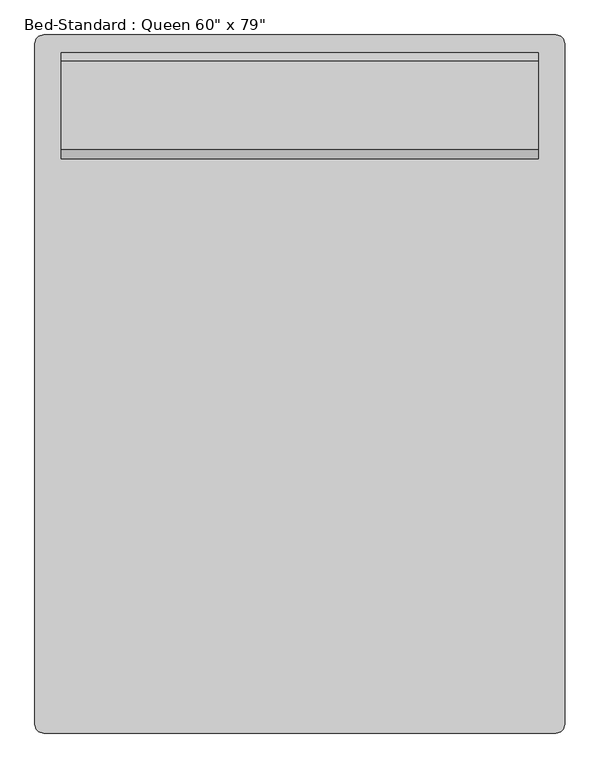
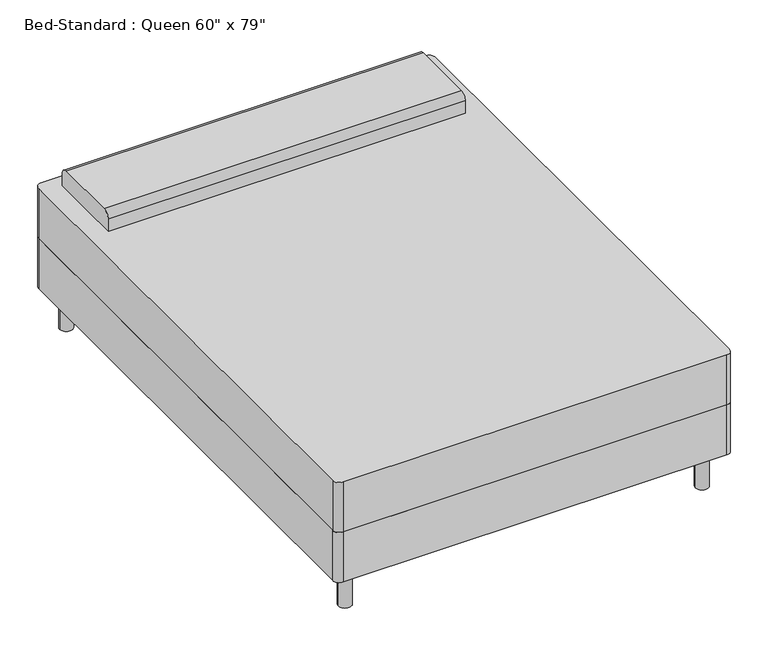
"""IFC4 building model written with IfcOpenShell, lengths in millimetres: furniture geometry."""

from ifc_helpers import new_model, si_unit, point, frame, frame_2d, origin, origin_with_axes, place, context, project, spatial, polyline, circle_curve, trimmed, segment, composite_curve, outline, extrude, source, transform, mapped, element, save


def furniture_e1791683(model_context):
    return source(origin(), model_context, "Body", "SweptSolid", [
        extrude(outline(composite_curve([segment(polyline([(-490.5114754, -1023.495082), (-490.5114754, 932.304918)]), True, "CONTINUOUS"), segment(trimmed(circle_curve(frame_2d((-465.1114754, 932.304918)), 25.4), [point((-490.5114754, 932.304918))], [point((-465.1114754, 957.704918))], False, "CARTESIAN"), True, "CONTINUOUS"), segment(polyline([(-465.1114754, 957.704918), (1008.0885246, 957.704918)]), True, "CONTINUOUS"), segment(trimmed(circle_curve(frame_2d((1008.0885246, 932.304918)), 25.4), [point((1008.0885246, 957.704918))], [point((1033.4885246, 932.304918))], False, "CARTESIAN"), True, "CONTINUOUS"), segment(polyline([(1033.4885246, 932.304918), (1033.4885246, -1023.495082)]), True, "CONTINUOUS"), segment(trimmed(circle_curve(frame_2d((1008.0885246, -1023.495082)), 25.4), [point((1033.4885246, -1023.495082))], [point((1008.0885246, -1048.895082))], False, "CARTESIAN"), True, "CONTINUOUS"), segment(polyline([(1008.0885246, -1048.895082), (-465.1114754, -1048.895082)]), True, "CONTINUOUS"), segment(trimmed(circle_curve(frame_2d((-465.1114754, -1023.495082)), 25.4), [point((-465.1114754, -1048.895082))], [point((-490.5114754, -1023.495082))], False, "CARTESIAN"), True, "CONTINUOUS")], self_intersect=False)), frame((0.0, 0.0, 152.4), z_axis=(0.0, 0.0, 1.0), x_axis=(1.0, 0.0, 0.0)), (0.0, 0.0, 1.0), 203.2),
        extrude(outline(composite_curve([segment(polyline([(602.104918, 558.8), (602.104918, 609.6)]), True, "CONTINUOUS"), segment(trimmed(circle_curve(frame_2d((627.504918, 609.6)), 25.4), [point((602.104918, 609.6))], [point((627.504918, 635.0))], False, "CARTESIAN"), True, "CONTINUOUS"), segment(polyline([(627.504918, 635.0), (881.504918, 635.0)]), True, "CONTINUOUS"), segment(trimmed(circle_curve(frame_2d((881.504918, 609.6)), 25.4), [point((881.504918, 635.0))], [point((906.904918, 609.6))], False, "CARTESIAN"), True, "CONTINUOUS"), segment(polyline([(906.904918, 609.6), (906.904918, 558.8), (602.104918, 558.8)]), True, "CONTINUOUS")], self_intersect=False)), frame((-414.3114754, 0.0, 0.0), z_axis=(1.0, 0.0, 0.0), x_axis=(0.0, 1.0, 0.0)), (0.0, 0.0, 1.0), 1371.6),
        extrude(outline(composite_curve([segment(trimmed(circle_curve(frame_2d((-414.3114754, 881.504918)), 25.4), [point((-439.7114754, 881.504918))], [point((-388.9114754, 881.504918))], False, "CARTESIAN"), True, "CONTINUOUS"), segment(trimmed(circle_curve(frame_2d((-414.3114754, 881.504918)), 25.4), [point((-388.9114754, 881.504918))], [point((-439.7114754, 881.504918))], False, "CARTESIAN"), True, "CONTINUOUS")], self_intersect=False)), origin_with_axes(), (0.0, 0.0, 1.0), 152.4),
        extrude(outline(composite_curve([segment(trimmed(circle_curve(frame_2d((957.2885246, 881.504918)), 25.4), [point((931.8885246, 881.504918))], [point((982.6885246, 881.504918))], False, "CARTESIAN"), True, "CONTINUOUS"), segment(trimmed(circle_curve(frame_2d((957.2885246, 881.504918)), 25.4), [point((982.6885246, 881.504918))], [point((931.8885246, 881.504918))], False, "CARTESIAN"), True, "CONTINUOUS")], self_intersect=False)), origin_with_axes(), (0.0, 0.0, 1.0), 152.4),
        extrude(outline(composite_curve([segment(trimmed(circle_curve(frame_2d((957.2885246, -972.695082)), 25.4), [point((931.8885246, -972.695082))], [point((982.6885246, -972.695082))], False, "CARTESIAN"), True, "CONTINUOUS"), segment(trimmed(circle_curve(frame_2d((957.2885246, -972.695082)), 25.4), [point((982.6885246, -972.695082))], [point((931.8885246, -972.695082))], False, "CARTESIAN"), True, "CONTINUOUS")], self_intersect=False)), origin_with_axes(), (0.0, 0.0, 1.0), 152.4),
        extrude(outline(composite_curve([segment(trimmed(circle_curve(frame_2d((-414.3114754, -972.695082)), 25.4), [point((-439.7114754, -972.695082))], [point((-388.9114754, -972.695082))], False, "CARTESIAN"), True, "CONTINUOUS"), segment(trimmed(circle_curve(frame_2d((-414.3114754, -972.695082)), 25.4), [point((-388.9114754, -972.695082))], [point((-439.7114754, -972.695082))], False, "CARTESIAN"), True, "CONTINUOUS")], self_intersect=False)), origin_with_axes(), (0.0, 0.0, 1.0), 152.4),
        extrude(outline(composite_curve([segment(polyline([(-465.1114754, 957.704918), (1008.0885246, 957.704918)]), True, "CONTINUOUS"), segment(trimmed(circle_curve(frame_2d((1008.0885246, 932.304918)), 25.4), [point((1008.0885246, 957.704918))], [point((1033.4885246, 932.304918))], False, "CARTESIAN"), True, "CONTINUOUS"), segment(polyline([(1033.4885246, 932.304918), (1033.4885246, -1023.495082)]), True, "CONTINUOUS"), segment(trimmed(circle_curve(frame_2d((1008.0885246, -1023.495082)), 25.4), [point((1033.4885246, -1023.495082))], [point((1008.0885246, -1048.895082))], False, "CARTESIAN"), True, "CONTINUOUS"), segment(polyline([(1008.0885246, -1048.895082), (-465.1114754, -1048.895082)]), True, "CONTINUOUS"), segment(trimmed(circle_curve(frame_2d((-465.1114754, -1023.495082)), 25.4), [point((-465.1114754, -1048.895082))], [point((-490.5114754, -1023.495082))], False, "CARTESIAN"), True, "CONTINUOUS"), segment(polyline([(-490.5114754, -1023.495082), (-490.5114754, 932.304918)]), True, "CONTINUOUS"), segment(trimmed(circle_curve(frame_2d((-465.1114754, 932.304918)), 25.4), [point((-490.5114754, 932.304918))], [point((-465.1114754, 957.704918))], False, "CARTESIAN"), True, "CONTINUOUS")], self_intersect=False)), frame((0.0, 0.0, 355.6), z_axis=(0.0, 0.0, 1.0), x_axis=(1.0, 0.0, 0.0)), (0.0, 0.0, 1.0), 203.2),
    ])


if __name__ == "__main__":
    model = new_model("IFC4")
    model_context = context("Model", 3, world=origin())
    ifc_project = project(units=[si_unit("LENGTHUNIT", "METRE", prefix="MILLI")], contexts=[model_context])
    site = spatial("IfcSite", under=ifc_project)
    building = spatial("IfcBuilding", under=site)
    placement = place(None, origin())
    furniture_shape = furniture_e1791683(model_context)
    element("IfcFurniture", 1, ObjectType="Bed-Standard : Queen 60\" x 79\"", at=placement, inside=building, context=model_context, shape_type="MappedRepresentation", body=[
        mapped(furniture_shape, transform((0.0, 0.0, 0.0), x_axis=(1.0, 0.0, 0.0), y_axis=(0.0, 1.0, 0.0), z_axis=(0.0, 0.0, 1.0))),
    ])
    save(model, "model.ifc")

# Revit data of these elements
# Type "Bed-Standard : Queen 60\" x 79\""
#   Assembly Code = "E2020200"
#   Length = 6' - 7"
#   Width = 5' - 0"
#   Leg Material = Steel, Chrome Plated
#   Mattress Material = Plywood, Sheathing
#   Default Elevation = 0
# Element 1 (IfcFurniture, "Bed-Standard : Queen 60\" x 79\"")
#   Materials on its faces: "Linen, White", "Steel, Chrome Plated"
# Materials
#   "Steel, Chrome Plated": class "Metal", colour RGB 17 17 17, transparency 0, Description = "Chromiuim plated steel", Cost = 0
#   "Plywood, Sheathing": class "Wood", colour RGB 212 179 113, transparency 0, Description = "Plywood, sheathing grade", Cost = 0
#   "Linen, White": class "Textile", colour RGB 247 247 239, transparency 0, Description = "Linen, white", Cost = 0
